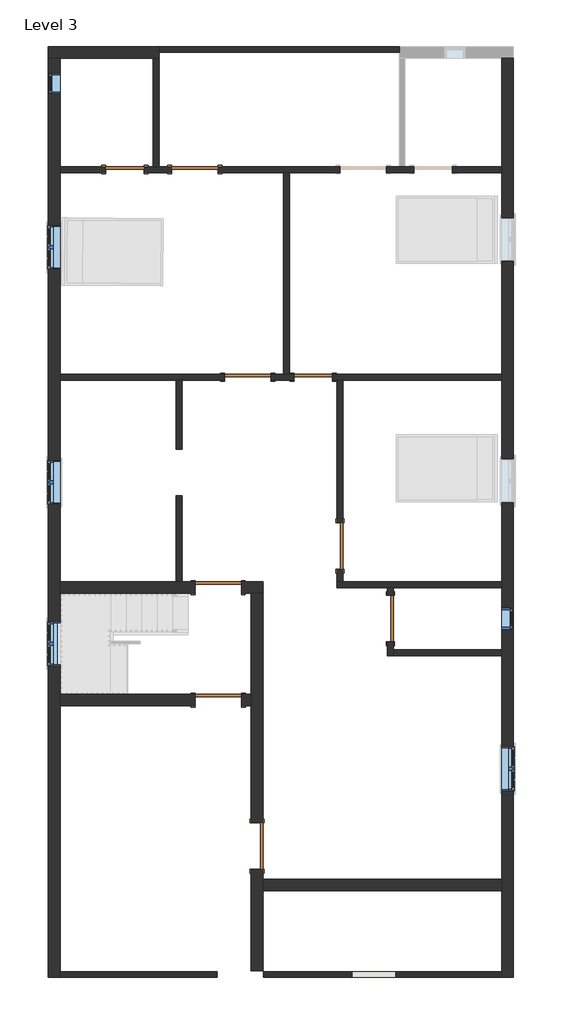
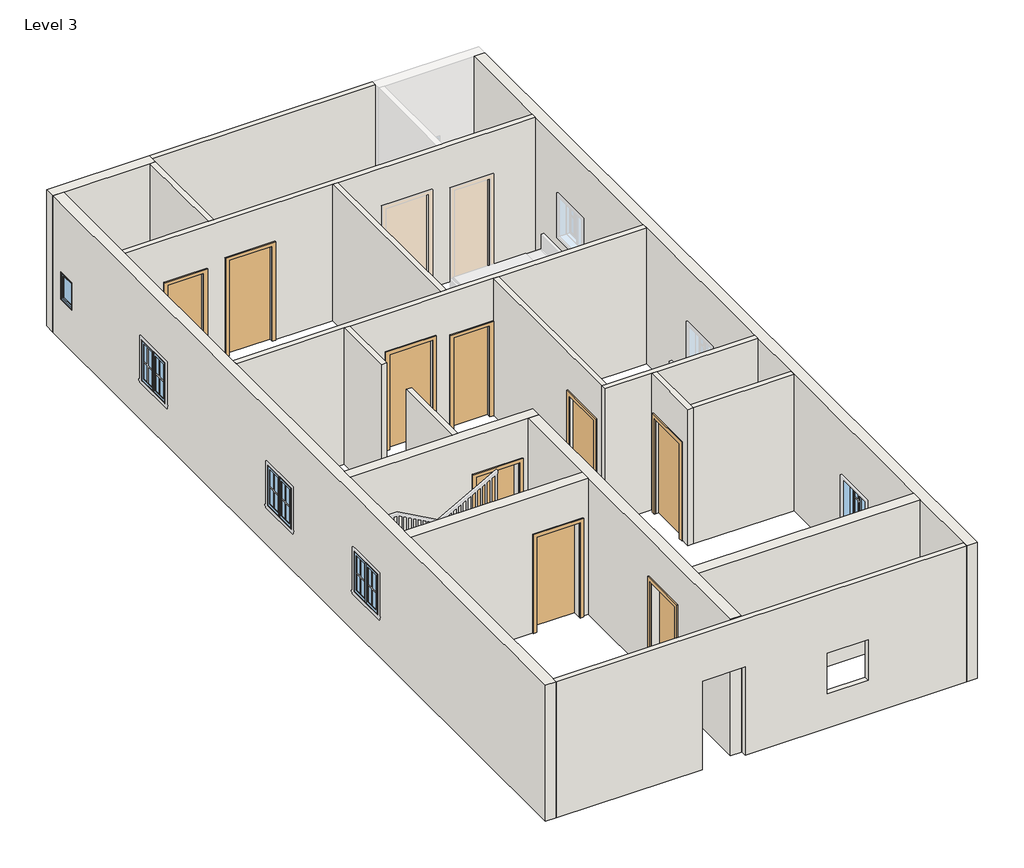
# One storey, part 1 of 3: 19 walls, 9 doors, 6 windows.
"""IFC4 building model written with IfcOpenShell, lengths in millimetres."""

from ifc_helpers import new_model, si_unit, frame, origin, place, context, project, spatial, polyline, outline, extrude, faceted_brep, transform, mapped, element, save
from components import door_d8f5dbb5, door_f2b275c1, door_e5f9f3c4, door_0ca8825f, door_305aa2a5, window_aa618e30, window_339605e1

model = new_model("IFC4")

# Units and contexts
model_context = context("Model", 3, world=origin())
ifc_project = project(units=[si_unit("LENGTHUNIT", "METRE", prefix="MILLI")], contexts=[model_context])

# Site, building, storey
site = spatial("IfcSite", under=ifc_project)
building = spatial("IfcBuilding", under=site)
storey = spatial("IfcBuildingStorey", under=building, Name="Level 3", Elevation=3200.4)

# Doors
placement = place(None, origin())
door_shape = door_d8f5dbb5(model_context)
element("IfcDoor", 1, ObjectType="Single-Flush : 30\" x 80\"", at=placement, inside=storey, context=model_context, shape_type="MappedRepresentation", body=[
    mapped(door_shape, transform((-4322.2915084, 8007.7072267, 3200.4), x_axis=(1.0, 0.0, 0.0), y_axis=(0.0, 1.0, 0.0), z_axis=(0.0, 0.0, 1.0))),
])
door_2_shape = door_f2b275c1(model_context)
element("IfcDoor", 2, ObjectType="Single-Flush : 30\" x 80\"", at=placement, inside=storey, context=model_context, shape_type="MappedRepresentation", body=[
    mapped(door_2_shape, transform((-621.124692, 3931.0072267, 3200.4), x_axis=(-1.0, 0.0, 0.0), y_axis=(0.0, -1.0, 0.0), z_axis=(0.0, 0.0, 1.0))),
])
door_3_shape = door_e5f9f3c4(model_context)
element("IfcDoor", 3, ObjectType="Single-Flush : 36\" x 84\"", at=placement, inside=storey, context=model_context, shape_type="MappedRepresentation", body=[
    mapped(door_3_shape, transform((-1909.2915084, 3931.0072267, 3200.4), x_axis=(1.0, 0.0, 0.0), y_axis=(0.0, 1.0, 0.0), z_axis=(0.0, 0.0, 1.0))),
])
element("IfcDoor", 4, ObjectType="Single-Flush : 36\" x 84\"", at=placement, inside=storey, context=model_context, shape_type="MappedRepresentation", body=[
    mapped(door_3_shape, transform((-94.9578757, 616.3072267, 3200.4), x_axis=(0.0, -1.0, 0.0), y_axis=(1.0, 0.0, 0.0), z_axis=(0.0, 0.0, 1.0))),
])
door_4_shape = door_0ca8825f(model_context)
element("IfcDoor", 5, ObjectType="Single-Flush : 36\" x 84\"", at=placement, inside=storey, context=model_context, shape_type="MappedRepresentation", body=[
    mapped(door_4_shape, transform((-2490.3165084, -202.8427733, 3200.4), x_axis=(1.0, 0.0, 0.0), y_axis=(0.0, 1.0, 0.0), z_axis=(0.0, 0.0, 1.0))),
])
element("IfcDoor", 6, ObjectType="Single-Flush : 36\" x 84\"", at=placement, inside=storey, context=model_context, shape_type="MappedRepresentation", body=[
    mapped(door_4_shape, transform((-2487.1415084, -2412.6427733, 3200.4), x_axis=(1.0, 0.0, 0.0), y_axis=(0.0, 1.0, 0.0), z_axis=(0.0, 0.0, 1.0))),
])
element("IfcDoor", 7, ObjectType="Single-Flush : 36\" x 84\"", at=placement, inside=storey, context=model_context, shape_type="MappedRepresentation", body=[
    mapped(door_4_shape, transform((-1725.1415084, -5282.8427733, 3200.4), x_axis=(0.0, -1.0, 0.0), y_axis=(1.0, 0.0, 0.0), z_axis=(0.0, 0.0, 1.0))),
])
door_5_shape = door_305aa2a5(model_context)
element("IfcDoor", 8, ObjectType="Single-Flush : 36\" x 84\"", at=placement, inside=storey, context=model_context, shape_type="MappedRepresentation", body=[
    mapped(door_5_shape, transform((897.4084916, -812.4427733, 3200.4), x_axis=(0.0, 1.0, 0.0), y_axis=(-1.0, 0.0, 0.0), z_axis=(0.0, 0.0, 1.0))),
])
element("IfcDoor", 9, ObjectType="Single-Flush : 36\" x 84\"", at=placement, inside=storey, context=model_context, shape_type="MappedRepresentation", body=[
    mapped(door_5_shape, transform((-2950.6915084, 8007.7072267, 3200.4), x_axis=(-1.0, 0.0, 0.0), y_axis=(0.0, -1.0, 0.0), z_axis=(0.0, 0.0, 1.0))),
])

# Walls
element("IfcWall", 10, ObjectType="WALL4.5\"", at=placement, inside=storey, context=model_context, shape_type="Brep", body=[
    faceted_brep([(821.2084916, 7950.5572267, 5334.0), (821.2084916, 7950.5572267, 3200.4), (1354.6084916, 7950.5572267, 3200.4), (1354.6084916, 7950.5572267, 5232.4), (2116.6084916, 7950.5572267, 5232.4), (2116.6084916, 7950.5572267, 3200.4), (3088.1584916, 7950.5572267, 3200.4), (3088.1584916, 7950.5572267, 6248.4), (-1090.1415084, 7950.5572267, 6248.4), (-1204.4415084, 7950.5572267, 6248.4), (-5598.6415084, 7950.5572267, 6248.4), (-5598.6415084, 7950.5572267, 3200.4), (-4703.2915084, 7950.5572267, 3200.4), (-4703.2915084, 7950.5572267, 5232.4), (-3941.2915084, 7950.5572267, 5232.4), (-3941.2915084, 7950.5572267, 3200.4), (-3407.8915084, 7950.5572267, 3200.4), (-3407.8915084, 7950.5572267, 5334.0), (-2493.4915084, 7950.5572267, 5334.0), (-2493.4915084, 7950.5572267, 3200.4), (-1204.4415084, 7950.5572267, 3200.4), (-1090.1415084, 7950.5572267, 3200.4), (-93.1915084, 7950.5572267, 3200.4), (-93.1915084, 7950.5572267, 5334.0), (1354.6084916, 8064.8572267, 3200.4), (1183.1584916, 8064.8572267, 3200.4), (1068.8584916, 8064.8572267, 3200.4), (821.2084916, 8064.8572267, 3200.4), (821.2084916, 8064.8572267, 5334.0), (-93.1915084, 8064.8572267, 5334.0), (-93.1915084, 8064.8572267, 3200.4), (-2493.4915084, 8064.8572267, 3200.4), (-2493.4915084, 8064.8572267, 5334.0), (-3407.8915084, 8064.8572267, 5334.0), (-3407.8915084, 8064.8572267, 3200.4), (-3655.5415084, 8064.8572267, 3200.4), (-3769.8415084, 8064.8572267, 3200.4), (-3941.2915084, 8064.8572267, 3200.4), (-3941.2915084, 8064.8572267, 5232.4), (-4703.2915084, 8064.8572267, 5232.4), (-4703.2915084, 8064.8572267, 3200.4), (-5598.6415084, 8064.8572267, 3200.4), (-5598.6415084, 8064.8572267, 6248.4), (-3769.8415084, 8064.8572267, 6248.4), (-3655.5415084, 8064.8572267, 6248.4), (1068.8584916, 8064.8572267, 6248.4), (1183.1584916, 8064.8572267, 6248.4), (3088.1584916, 8064.8572267, 6248.4), (3088.1584916, 8064.8572267, 3200.4), (2116.6084916, 8064.8572267, 3200.4), (2116.6084916, 8064.8572267, 5232.4), (1354.6084916, 8064.8572267, 5232.4)], [[[0, 1, 2, 3, 4, 5, 6, 7, 8, 9, 10, 11, 12, 13, 14, 15, 16, 17, 18, 19, 20, 21, 22, 23]], [[24, 25, 26, 27, 28, 29, 30, 31, 32, 33, 34, 35, 36, 37, 38, 39, 40, 41, 42, 43, 44, 45, 46, 47, 48, 49, 50, 51]], [[12, 11, 41, 40]], [[49, 48, 6, 5]], [[37, 36, 35, 34, 16, 15]], [[2, 1, 27, 26, 25, 24]], [[22, 21, 20, 19, 31, 30]], [[11, 10, 42, 41]], [[7, 6, 48, 47]], [[38, 37, 15, 14]], [[39, 38, 14, 13]], [[40, 39, 13, 12]], [[3, 2, 24, 51]], [[4, 3, 51, 50]], [[5, 4, 50, 49]], [[17, 16, 34, 33]], [[18, 17, 33, 32]], [[19, 18, 32, 31]], [[28, 27, 1, 0]], [[29, 28, 0, 23]], [[30, 29, 23, 22]], [[10, 9, 8, 7, 47, 46, 45, 44, 43, 42]]]),
])
element("IfcWall", 11, ObjectType="WALL4.5\"", at=placement, inside=storey, context=model_context, shape_type="SweptSolid", body=[
    extrude(outline(polyline([(-3769.8415084, 8064.8572267), (-3769.8415084, 10198.4572267), (-3655.5415084, 10198.4572267), (-3655.5415084, 8064.8572267), (-3769.8415084, 8064.8572267)])), frame((0.0, 0.0, 3200.4), z_axis=(0.0, 0.0, 1.0), x_axis=(1.0, 0.0, 0.0)), (0.0, 0.0, 1.0), 3048.0),
])
element("IfcWall", 12, ObjectType="WALL4.5\"", at=placement, inside=storey, context=model_context, shape_type="SweptSolid", body=[
    extrude(outline(polyline([(-1204.4415084, 3988.1572267), (-1204.4415084, 7950.5572267), (-1090.1415084, 7950.5572267), (-1090.1415084, 3988.1572267), (-1204.4415084, 3988.1572267)])), frame((0.0, 0.0, 3200.4), z_axis=(0.0, 0.0, 1.0), x_axis=(1.0, 0.0, 0.0)), (0.0, 0.0, 1.0), 3048.0),
])
element("IfcWall", 13, ObjectType="WALL4.5\"", at=placement, inside=storey, context=model_context, shape_type="Brep", body=[
    faceted_brep([(-1452.0915084, 3873.8572267, 3200.4), (-1002.124692, 3873.8572267, 3200.4), (-1002.124692, 3873.8572267, 5232.4), (-240.124692, 3873.8572267, 5232.4), (-240.124692, 3873.8572267, 3200.4), (-152.1078757, 3873.8572267, 3200.4), (-37.8078757, 3873.8572267, 3200.4), (3088.1584916, 3873.8572267, 3200.4), (3088.1584916, 3873.8572267, 6248.4), (-37.8078757, 3873.8572267, 6248.4), (-152.1078757, 3873.8572267, 6248.4), (-3198.3415084, 3873.8572267, 6248.4), (-3312.6415084, 3873.8572267, 6248.4), (-5598.6415084, 3873.8572267, 6248.4), (-5598.6415084, 3873.8572267, 3200.4), (-3312.6415084, 3873.8572267, 3200.4), (-3198.3415084, 3873.8572267, 3200.4), (-2366.4915084, 3873.8572267, 3200.4), (-2366.4915084, 3873.8572267, 5334.0), (-1452.0915084, 3873.8572267, 5334.0), (-1002.124692, 3988.1572267, 5232.4), (-1002.124692, 3988.1572267, 3200.4), (-1090.1415084, 3988.1572267, 3200.4), (-1204.4415084, 3988.1572267, 3200.4), (-1452.0915084, 3988.1572267, 3200.4), (-1452.0915084, 3988.1572267, 5334.0), (-2366.4915084, 3988.1572267, 5334.0), (-2366.4915084, 3988.1572267, 3200.4), (-5598.6415084, 3988.1572267, 3200.4), (-5598.6415084, 3988.1572267, 6248.4), (-1204.4415084, 3988.1572267, 6248.4), (-1090.1415084, 3988.1572267, 6248.4), (3088.1584916, 3988.1572267, 6248.4), (3088.1584916, 3988.1572267, 3200.4), (-240.124692, 3988.1572267, 3200.4), (-240.124692, 3988.1572267, 5232.4)], [[[0, 1, 2, 3, 4, 5, 6, 7, 8, 9, 10, 11, 12, 13, 14, 15, 16, 17, 18, 19]], [[20, 21, 22, 23, 24, 25, 26, 27, 28, 29, 30, 31, 32, 33, 34, 35]], [[17, 16, 15, 14, 28, 27]], [[34, 33, 7, 6, 5, 4]], [[24, 23, 22, 21, 1, 0]], [[14, 13, 29, 28]], [[8, 7, 33, 32]], [[25, 24, 0, 19]], [[26, 25, 19, 18]], [[27, 26, 18, 17]], [[2, 1, 21, 20]], [[3, 2, 20, 35]], [[4, 3, 35, 34]], [[13, 12, 11, 10, 9, 8, 32, 31, 30, 29]]]),
])
element("IfcWall", 14, ObjectType="WALL4.5\"", at=placement, inside=storey, context=model_context, shape_type="SweptSolid", body=[
    extrude(outline(polyline([(-3312.6415084, 2514.5843832), (-3312.6415084, 3873.8572267), (-3198.3415084, 3873.8572267), (-3198.3415084, 2514.5843832), (-3312.6415084, 2514.5843832)])), frame((0.0, 0.0, 3200.4), z_axis=(0.0, 0.0, 1.0), x_axis=(1.0, 0.0, 0.0)), (0.0, 0.0, 1.0), 3048.0),
])
element("IfcWall", 15, ObjectType="WALL4.5\"", at=placement, inside=storey, context=model_context, shape_type="SweptSolid", body=[
    extrude(outline(polyline([(-3312.6415084, -88.5427733), (-3312.6415084, 1600.2092553), (-3198.3415084, 1600.2092553), (-3198.3415084, -88.5427733), (-3312.6415084, -88.5427733)])), frame((0.0, 0.0, 3200.4), z_axis=(0.0, 0.0, 1.0), x_axis=(1.0, 0.0, 0.0)), (0.0, 0.0, 1.0), 3048.0),
])
element("IfcWall", 16, ObjectType="WALL4.5\"", at=placement, inside=storey, context=model_context, shape_type="SweptSolid", body=[
    extrude(outline(polyline([(159.1072267, 5334.0), (159.1072267, 3200.4), (-88.5427733, 3200.4), (-88.5427733, 6248.4), (3873.8572267, 6248.4), (3873.8572267, 3200.4), (1073.5072267, 3200.4), (1073.5072267, 5334.0), (159.1072267, 5334.0)])), frame((-152.1078757, 0.0, 0.0), z_axis=(1.0, 0.0, 0.0), x_axis=(0.0, 1.0, 0.0)), (0.0, 0.0, 1.0), 114.3),
])
element("IfcWall", 17, ObjectType="WALL4.5\"", at=placement, inside=storey, context=model_context, shape_type="Brep", body=[
    faceted_brep([(-152.1078757, -202.8427733, 3200.4), (840.2584916, -202.8427733, 3200.4), (954.5584916, -202.8427733, 3200.4), (3088.1584916, -202.8427733, 3200.4), (3088.1584916, -202.8427733, 6248.4), (954.5584916, -202.8427733, 6248.4), (840.2584916, -202.8427733, 6248.4), (-152.1078757, -202.8427733, 6248.4), (-152.1078757, -88.5427733, 3200.4), (-152.1078757, -88.5427733, 6248.4), (-37.8078757, -88.5427733, 6248.4), (3088.1584916, -88.5427733, 6248.4), (3088.1584916, -88.5427733, 3200.4), (-37.8078757, -88.5427733, 3200.4)], [[[0, 1, 2, 3, 4, 5, 6, 7]], [[8, 9, 10, 11, 12, 13]], [[3, 2, 1, 0, 8, 13, 12]], [[4, 3, 12, 11]], [[0, 7, 9, 8]], [[7, 6, 5, 4, 11, 10, 9]]]),
])
element("IfcWall", 18, ObjectType="WALL4.5\"", at=placement, inside=storey, context=model_context, shape_type="Brep", body=[
    faceted_brep([(840.2584916, -202.8427733, 3200.4), (840.2584916, -355.2427733, 3200.4), (840.2584916, -355.2427733, 5334.0), (840.2584916, -1269.6427733, 5334.0), (840.2584916, -1269.6427733, 3200.4), (840.2584916, -1536.3427733, 3200.4), (840.2584916, -1536.3427733, 6248.4), (840.2584916, -202.8427733, 6248.4), (954.5584916, -355.2427733, 5334.0), (954.5584916, -355.2427733, 3200.4), (954.5584916, -202.8427733, 3200.4), (954.5584916, -202.8427733, 6248.4), (954.5584916, -1422.0427733, 6248.4), (954.5584916, -1536.3427733, 6248.4), (954.5584916, -1536.3427733, 3200.4), (954.5584916, -1422.0427733, 3200.4), (954.5584916, -1269.6427733, 3200.4), (954.5584916, -1269.6427733, 5334.0)], [[[0, 1, 2, 3, 4, 5, 6, 7]], [[8, 9, 10, 11, 12, 13, 14, 15, 16, 17]], [[10, 9, 1, 0]], [[16, 15, 14, 5, 4]], [[0, 7, 11, 10]], [[6, 5, 14, 13]], [[2, 1, 9, 8]], [[3, 2, 8, 17]], [[4, 3, 17, 16]], [[7, 6, 13, 12, 11]]]),
])
element("IfcWall", 19, ObjectType="WALL4.5\"", at=placement, inside=storey, context=model_context, shape_type="SweptSolid", body=[
    extrude(outline(polyline([(3088.1584916, -1536.3427733), (954.5584916, -1536.3427733), (954.5584916, -1422.0427733), (3088.1584916, -1422.0427733), (3088.1584916, -1536.3427733)])), frame((0.0, 0.0, 3200.4), z_axis=(0.0, 0.0, 1.0), x_axis=(1.0, 0.0, 0.0)), (0.0, 0.0, 1.0), 3048.0),
])
element("IfcWall", 20, ObjectType="WALL4.5\"", at=placement, inside=storey, context=model_context, shape_type="SweptSolid", body=[
    extrude(outline(polyline([(6248.4, -5598.6415084), (3200.4, -5598.6415084), (3200.4, -2512.5415084), (5181.6, -2512.5415084), (5181.6, -1598.1415084), (3200.4, -1598.1415084), (3200.4, 3088.1584916), (6248.4, 3088.1584916), (6248.4, -5598.6415084)]), holes=[polyline([(4876.8, 141.7584916), (4876.8, 1005.3584916), (3962.4, 1005.3584916), (3962.4, 141.7584916), (4876.8, 141.7584916)])]), frame((0.0, -7860.9427733, 0.0), z_axis=(0.0, 1.0, 0.0), x_axis=(0.0, 0.0, 1.0)), (0.0, 0.0, 1.0), 114.3),
])
element("IfcWall", 21, ObjectType="WALL4.5\"", at=placement, inside=storey, context=model_context, shape_type="SweptSolid", body=[
    extrude(outline(polyline([(1068.8584916, 10312.7572267), (-3655.5415084, 10312.7572267), (-3655.5415084, 10427.0572267), (1068.8584916, 10427.0572267), (1068.8584916, 10312.7572267)])), frame((0.0, 0.0, 3200.4), z_axis=(0.0, 0.0, 1.0), x_axis=(1.0, 0.0, 0.0)), (0.0, 0.0, 1.0), 3048.0),
])
element("IfcWall", 22, ObjectType="WALL9\"", at=placement, inside=storey, context=model_context, shape_type="Brep", body=[
    faceted_brep([(-3655.5415084, 10427.0572267, 3200.4), (-5827.2415084, 10427.0572267, 3200.4), (-5827.2415084, 10427.0572267, 6248.4), (-3655.5415084, 10427.0572267, 6248.4), (-3655.5415084, 10198.4572267, 3200.4), (-3655.5415084, 10198.4572267, 6248.4), (-3769.8415084, 10198.4572267, 6248.4), (-5598.6415084, 10198.4572267, 6248.4), (-5827.2415084, 10198.4572267, 6248.4), (-5827.2415084, 10198.4572267, 3200.4), (-5598.6415084, 10198.4572267, 3200.4), (-3769.8415084, 10198.4572267, 3200.4), (-3655.5415084, 10312.7572267, 3200.4), (-3655.5415084, 10312.7572267, 6248.4)], [[[0, 1, 2, 3]], [[4, 5, 6, 7, 8, 9, 10, 11]], [[1, 0, 12, 4, 11, 10, 9]], [[2, 1, 9, 8]], [[0, 3, 13, 5, 4, 12]], [[3, 2, 8, 7, 6, 5, 13]]]),
])
element("IfcWall", 23, ObjectType="WALL9\"", at=placement, inside=storey, context=model_context, shape_type="Brep", body=[
    faceted_brep([(-5827.2415084, 10198.4572267, 3200.4), (-5827.2415084, -7860.9427733, 3200.4), (-5827.2415084, -7860.9427733, 6248.4), (-5827.2415084, 10198.4572267, 6248.4), (-5827.2415084, 9906.3572267, 4724.4), (-5827.2415084, 9499.9572267, 4724.4), (-5827.2415084, 9499.9572267, 4114.8), (-5827.2415084, 9906.3572267, 4114.8), (-5827.2415084, 6915.5072267, 5029.2), (-5827.2415084, 6051.9072267, 5029.2), (-5827.2415084, 6051.9072267, 4114.8), (-5827.2415084, 6915.5072267, 4114.8), (-5827.2415084, 2295.8822267, 5029.2), (-5827.2415084, 1432.2822267, 5029.2), (-5827.2415084, 1432.2822267, 4114.8), (-5827.2415084, 2295.8822267, 4114.8), (-5827.2415084, -875.9427733, 5029.2), (-5827.2415084, -1739.5427733, 5029.2), (-5827.2415084, -1739.5427733, 4114.8), (-5827.2415084, -875.9427733, 4114.8), (-5598.6415084, 10198.4572267, 3200.4), (-5598.6415084, 10198.4572267, 6248.4), (-5598.6415084, 8064.8572267, 6248.4), (-5598.6415084, 7950.5572267, 6248.4), (-5598.6415084, 3988.1572267, 6248.4), (-5598.6415084, 3873.8572267, 6248.4), (-5598.6415084, -88.5427733, 6248.4), (-5598.6415084, -317.1427733, 6248.4), (-5598.6415084, -2298.3427733, 6248.4), (-5598.6415084, -2526.9427733, 6248.4), (-5598.6415084, -7746.6427733, 6248.4), (-5598.6415084, -7860.9427733, 6248.4), (-5598.6415084, -7860.9427733, 3200.4), (-5598.6415084, -7746.6427733, 3200.4), (-5598.6415084, -2526.9427733, 3200.4), (-5598.6415084, -2298.3427733, 3200.4), (-5598.6415084, -317.1427733, 3200.4), (-5598.6415084, -88.5427733, 3200.4), (-5598.6415084, 3873.8572267, 3200.4), (-5598.6415084, 3988.1572267, 3200.4), (-5598.6415084, 7950.5572267, 3200.4), (-5598.6415084, 8064.8572267, 3200.4), (-5598.6415084, 9906.3572267, 4724.4), (-5598.6415084, 9906.3572267, 4114.8), (-5598.6415084, 9499.9572267, 4114.8), (-5598.6415084, 9499.9572267, 4724.4), (-5598.6415084, 6915.5072267, 5029.2), (-5598.6415084, 6915.5072267, 4114.8), (-5598.6415084, 6051.9072267, 4114.8), (-5598.6415084, 6051.9072267, 5029.2), (-5598.6415084, 2295.8822267, 5029.2), (-5598.6415084, 2295.8822267, 4114.8), (-5598.6415084, 1432.2822267, 4114.8), (-5598.6415084, 1432.2822267, 5029.2), (-5598.6415084, -875.9427733, 5029.2), (-5598.6415084, -875.9427733, 4114.8), (-5598.6415084, -1739.5427733, 4114.8), (-5598.6415084, -1739.5427733, 5029.2)], [[[0, 1, 2, 3], [4, 5, 6, 7], [8, 9, 10, 11], [12, 13, 14, 15], [16, 17, 18, 19]], [[20, 21, 22, 23, 24, 25, 26, 27, 28, 29, 30, 31, 32, 33, 34, 35, 36, 37, 38, 39, 40, 41], [42, 43, 44, 45], [46, 47, 48, 49], [50, 51, 52, 53], [54, 55, 56, 57]], [[1, 0, 20, 41, 40, 39, 38, 37, 36, 35, 34, 33, 32]], [[0, 3, 21, 20]], [[2, 1, 32, 31]], [[43, 42, 4, 7]], [[44, 43, 7, 6]], [[45, 44, 6, 5]], [[42, 45, 5, 4]], [[47, 46, 8, 11]], [[48, 47, 11, 10]], [[49, 48, 10, 9]], [[46, 49, 9, 8]], [[51, 50, 12, 15]], [[52, 51, 15, 14]], [[53, 52, 14, 13]], [[50, 53, 13, 12]], [[55, 54, 16, 19]], [[56, 55, 19, 18]], [[57, 56, 18, 17]], [[54, 57, 17, 16]], [[3, 2, 31, 30, 29, 28, 27, 26, 25, 24, 23, 22, 21]]]),
])
element("IfcWall", 24, ObjectType="WALL9\"", at=placement, inside=storey, context=model_context, shape_type="Brep", body=[
    faceted_brep([(3088.1584916, 10198.4572267, 3200.4), (3088.1584916, 8064.8572267, 3200.4), (3088.1584916, 7950.5572267, 3200.4), (3088.1584916, 3988.1572267, 3200.4), (3088.1584916, 3873.8572267, 3200.4), (3088.1584916, -88.5427733, 3200.4), (3088.1584916, -202.8427733, 3200.4), (3088.1584916, -1422.0427733, 3200.4), (3088.1584916, -1536.3427733, 3200.4), (3088.1584916, -5930.5427733, 3200.4), (3088.1584916, -6159.1427733, 3200.4), (3088.1584916, -7746.6427733, 3200.4), (3088.1584916, -7860.9427733, 3200.4), (3088.1584916, -7860.9427733, 6248.4), (3088.1584916, -7746.6427733, 6248.4), (3088.1584916, -6159.1427733, 6248.4), (3088.1584916, -5930.5427733, 6248.4), (3088.1584916, -1536.3427733, 6248.4), (3088.1584916, -1422.0427733, 6248.4), (3088.1584916, -202.8427733, 6248.4), (3088.1584916, -88.5427733, 6248.4), (3088.1584916, 3873.8572267, 6248.4), (3088.1584916, 3988.1572267, 6248.4), (3088.1584916, 7950.5572267, 6248.4), (3088.1584916, 8064.8572267, 6248.4), (3088.1584916, 10198.4572267, 6248.4), (3088.1584916, -1015.6427733, 4724.4), (3088.1584916, -1015.6427733, 4114.8), (3088.1584916, -609.2427733, 4114.8), (3088.1584916, -609.2427733, 4724.4), (3088.1584916, 6204.3072267, 5029.2), (3088.1584916, 6204.3072267, 4114.8), (3088.1584916, 7067.9072267, 4114.8), (3088.1584916, 7067.9072267, 5029.2), (3088.1584916, 1460.8572267, 5029.2), (3088.1584916, 1460.8572267, 4114.8), (3088.1584916, 2324.4572267, 4114.8), (3088.1584916, 2324.4572267, 5029.2), (3088.1584916, -4193.8177733, 5029.2), (3088.1584916, -4193.8177733, 4114.8), (3088.1584916, -3330.2177733, 4114.8), (3088.1584916, -3330.2177733, 5029.2), (3316.7584916, 10198.4572267, 3200.4), (3316.7584916, 10198.4572267, 6248.4), (3316.7584916, -7860.9427733, 6248.4), (3316.7584916, -7860.9427733, 3200.4), (3316.7584916, -1015.6427733, 4724.4), (3316.7584916, -609.2427733, 4724.4), (3316.7584916, -609.2427733, 4114.8), (3316.7584916, -1015.6427733, 4114.8), (3316.7584916, 6204.3072267, 5029.2), (3316.7584916, 7067.9072267, 5029.2), (3316.7584916, 7067.9072267, 4114.8), (3316.7584916, 6204.3072267, 4114.8), (3316.7584916, 1460.8572267, 5029.2), (3316.7584916, 2324.4572267, 5029.2), (3316.7584916, 2324.4572267, 4114.8), (3316.7584916, 1460.8572267, 4114.8), (3316.7584916, -4193.8177733, 5029.2), (3316.7584916, -3330.2177733, 5029.2), (3316.7584916, -3330.2177733, 4114.8), (3316.7584916, -4193.8177733, 4114.8)], [[[0, 1, 2, 3, 4, 5, 6, 7, 8, 9, 10, 11, 12, 13, 14, 15, 16, 17, 18, 19, 20, 21, 22, 23, 24, 25], [26, 27, 28, 29], [30, 31, 32, 33], [34, 35, 36, 37], [38, 39, 40, 41]], [[42, 43, 44, 45], [46, 47, 48, 49], [50, 51, 52, 53], [54, 55, 56, 57], [58, 59, 60, 61]], [[12, 11, 10, 9, 8, 7, 6, 5, 4, 3, 2, 1, 0, 42, 45]], [[0, 25, 43, 42]], [[13, 12, 45, 44]], [[27, 26, 46, 49]], [[28, 27, 49, 48]], [[29, 28, 48, 47]], [[26, 29, 47, 46]], [[31, 30, 50, 53]], [[32, 31, 53, 52]], [[33, 32, 52, 51]], [[30, 33, 51, 50]], [[35, 34, 54, 57]], [[36, 35, 57, 56]], [[37, 36, 56, 55]], [[34, 37, 55, 54]], [[39, 38, 58, 61]], [[40, 39, 61, 60]], [[41, 40, 60, 59]], [[38, 41, 59, 58]], [[25, 24, 23, 22, 21, 20, 19, 18, 17, 16, 15, 14, 13, 44, 43]]]),
])
element("IfcWall", 25, ObjectType="WALL9\"", at=placement, inside=storey, context=model_context, shape_type="Brep", body=[
    faceted_brep([(-2033.1165084, -317.1427733, 5334.0), (-2033.1165084, -317.1427733, 3200.4), (-1839.4415084, -317.1427733, 3200.4), (-1610.8415084, -317.1427733, 3200.4), (-1610.8415084, -317.1427733, 6248.4), (-1839.4415084, -317.1427733, 6248.4), (-5598.6415084, -317.1427733, 6248.4), (-5598.6415084, -317.1427733, 3200.4), (-2947.5165084, -317.1427733, 3200.4), (-2947.5165084, -317.1427733, 5334.0), (-1610.8415084, -88.5427733, 3200.4), (-2033.1165084, -88.5427733, 3200.4), (-2033.1165084, -88.5427733, 5334.0), (-2947.5165084, -88.5427733, 5334.0), (-2947.5165084, -88.5427733, 3200.4), (-3198.3415084, -88.5427733, 3200.4), (-3312.6415084, -88.5427733, 3200.4), (-5598.6415084, -88.5427733, 3200.4), (-5598.6415084, -88.5427733, 6248.4), (-3312.6415084, -88.5427733, 6248.4), (-3198.3415084, -88.5427733, 6248.4), (-1610.8415084, -88.5427733, 6248.4)], [[[0, 1, 2, 3, 4, 5, 6, 7, 8, 9]], [[10, 11, 12, 13, 14, 15, 16, 17, 18, 19, 20, 21]], [[8, 7, 17, 16, 15, 14]], [[3, 2, 1, 11, 10]], [[7, 6, 18, 17]], [[4, 3, 10, 21]], [[12, 11, 1, 0]], [[13, 12, 0, 9]], [[14, 13, 9, 8]], [[6, 5, 4, 21, 20, 19, 18]]]),
])
element("IfcWall", 26, ObjectType="WALL9\"", at=placement, inside=storey, context=model_context, shape_type="Brep", body=[
    faceted_brep([(-1839.4415084, -5740.0427733, 5334.0), (-1839.4415084, -5740.0427733, 3200.4), (-1839.4415084, -7733.9427733, 3200.4), (-1839.4415084, -7733.9427733, 6248.4), (-1839.4415084, -2526.9427733, 6248.4), (-1839.4415084, -2298.3427733, 6248.4), (-1839.4415084, -317.1427733, 6248.4), (-1839.4415084, -317.1427733, 3200.4), (-1839.4415084, -2298.3427733, 3200.4), (-1839.4415084, -2526.9427733, 3200.4), (-1839.4415084, -4825.6427733, 3200.4), (-1839.4415084, -4825.6427733, 5334.0), (-1610.8415084, -7733.9427733, 3200.4), (-1610.8415084, -6159.1427733, 3200.4), (-1610.8415084, -5930.5427733, 3200.4), (-1610.8415084, -5740.0427733, 3200.4), (-1610.8415084, -5740.0427733, 5334.0), (-1610.8415084, -4825.6427733, 5334.0), (-1610.8415084, -4825.6427733, 3200.4), (-1610.8415084, -317.1427733, 3200.4), (-1610.8415084, -317.1427733, 6248.4), (-1610.8415084, -5930.5427733, 6248.4), (-1610.8415084, -6159.1427733, 6248.4), (-1610.8415084, -7733.9427733, 6248.4)], [[[0, 1, 2, 3, 4, 5, 6, 7, 8, 9, 10, 11]], [[12, 13, 14, 15, 16, 17, 18, 19, 20, 21, 22, 23]], [[2, 1, 15, 14, 13, 12]], [[10, 9, 8, 7, 19, 18]], [[3, 2, 12, 23]], [[7, 6, 20, 19]], [[16, 15, 1, 0]], [[17, 16, 0, 11]], [[18, 17, 11, 10]], [[6, 5, 4, 3, 23, 22, 21, 20]]]),
])
element("IfcWall", 27, ObjectType="WALL9\"", at=placement, inside=storey, context=model_context, shape_type="SweptSolid", body=[
    extrude(outline(polyline([(3088.1584916, -6159.1427733), (-1610.8415084, -6159.1427733), (-1610.8415084, -5930.5427733), (3088.1584916, -5930.5427733), (3088.1584916, -6159.1427733)])), frame((0.0, 0.0, 3200.4), z_axis=(0.0, 0.0, 1.0), x_axis=(1.0, 0.0, 0.0)), (0.0, 0.0, 1.0), 3048.0),
])
element("IfcWall", 28, ObjectType="WALL9\"", at=placement, inside=storey, context=model_context, shape_type="SweptSolid", body=[
    extrude(outline(polyline([(5334.0, -2029.9415084), (3200.4, -2029.9415084), (3200.4, -1839.4415084), (6248.4, -1839.4415084), (6248.4, -5598.6415084), (3200.4, -5598.6415084), (3200.4, -2944.3415084), (5334.0, -2944.3415084), (5334.0, -2029.9415084)])), frame((0.0, -2526.9427733, 0.0), z_axis=(0.0, 1.0, 0.0), x_axis=(0.0, 0.0, 1.0)), (0.0, 0.0, 1.0), 228.6),
])

# Windows
window_shape = window_aa618e30(model_context)
element("IfcWindow", 29, ObjectType="Fixed : 16\" x 24\"", at=placement, inside=storey, context=model_context, shape_type="MappedRepresentation", body=[
    mapped(window_shape, transform((-5712.9415084, 9741.2572267, 3200.4), x_axis=(0.0, 1.0, 0.0), y_axis=(-1.0, 0.0, 0.0), z_axis=(0.0, 0.0, 1.0))),
])
element("IfcWindow", 30, ObjectType="Fixed : 16\" x 24\"", at=placement, inside=storey, context=model_context, shape_type="MappedRepresentation", body=[
    mapped(window_shape, transform((3202.4584916, -850.5427733, 3200.4), x_axis=(0.0, -1.0, 0.0), y_axis=(1.0, 0.0, 0.0), z_axis=(0.0, 0.0, 1.0))),
])
window_2_shape = window_339605e1(model_context)
element("IfcWindow", 31, ObjectType="Window-Casement-Double : 34\" x 36\"", at=placement, inside=storey, context=model_context, shape_type="MappedRepresentation", body=[
    mapped(window_2_shape, transform((-5712.9415084, 6483.7072267, 3200.4), x_axis=(0.0, 1.0, 0.0), y_axis=(-1.0, 0.0, 0.0), z_axis=(0.0, 0.0, 1.0))),
])
element("IfcWindow", 32, ObjectType="Window-Casement-Double : 34\" x 36\"", at=placement, inside=storey, context=model_context, shape_type="MappedRepresentation", body=[
    mapped(window_2_shape, transform((-5712.9415084, 1864.0822267, 3200.4), x_axis=(0.0, 1.0, 0.0), y_axis=(-1.0, 0.0, 0.0), z_axis=(0.0, 0.0, 1.0))),
])
element("IfcWindow", 33, ObjectType="Window-Casement-Double : 34\" x 36\"", at=placement, inside=storey, context=model_context, shape_type="MappedRepresentation", body=[
    mapped(window_2_shape, transform((3202.4584916, -3762.0177733, 3200.4), x_axis=(0.0, -1.0, 0.0), y_axis=(1.0, 0.0, 0.0), z_axis=(0.0, 0.0, 1.0))),
])
element("IfcWindow", 34, ObjectType="Window-Casement-Double : 34\" x 36\"", at=placement, inside=storey, context=model_context, shape_type="MappedRepresentation", body=[
    mapped(window_2_shape, transform((-5712.9415084, -1307.7427733, 3200.4), x_axis=(0.0, 1.0, 0.0), y_axis=(-1.0, 0.0, 0.0), z_axis=(0.0, 0.0, 1.0))),
])

save(model, "model.ifc")

# Revit data of these elements
# Type "Single-Flush : 30\" x 80\""
#   Type Mark = "5"
#   Construction Type Id = "MDOOR"
#   Assembly Code = "C1020"
#   Analytic Construction = "Metal"
#   Thickness = 0' - 2"
#   Heat Transfer Coefficient (U) = 0.651978 BTU/(h·ft²·°F)
#   Height = 6' - 8"
#   Trim Projection Ext = 0' - 1"
#   Trim Projection Int = 0' - 1"
#   Trim Width = 0' - 3"
#   Width = 2' - 6"
#   Define Thermal Properties by = 1
#   Define Thermal Properties by = 1
#   Door Material = Door - Panel
#   Frame Material = Door - Frame
#   Visual Light Transmittance = 0
#   Solar Heat Gain Coefficient = 0
#   Function = (empty or 0)
#   Wall Closure = (empty or 0)
# Type "Single-Flush : 36\" x 84\""
#   Type Mark = "1"
#   Construction Type Id = "MDOOR"
#   Assembly Code = "C1020"
#   Analytic Construction = "Metal"
#   Thickness = 0' - 2"
#   Heat Transfer Coefficient (U) = 0.651978 BTU/(h·ft²·°F)
#   Height = 7' - 0"
#   Trim Projection Ext = 0' - 1"
#   Trim Projection Int = 0' - 1"
#   Trim Width = 0' - 3"
#   Width = 3' - 0"
#   Define Thermal Properties by = 1
#   Define Thermal Properties by = 1
#   Door Material = Door - Panel
#   Frame Material = Door - Frame
#   Visual Light Transmittance = 0
#   Solar Heat Gain Coefficient = 0
#   Function = (empty or 0)
#   Wall Closure = (empty or 0)
# Type "WALL4.5\""
#   Assembly Code = "B2010"
#   Layers, outside or top first: 0' - 4 1/2" no material (function 1)
# Type "WALL9\""
#   Assembly Code = "B2010"
#   Layers, outside or top first: 0' - 9" no material (function 1)
# Type "Fixed : 16\" x 24\""
#   Type Mark = "4"
#   Construction Type Id = "GSP4R"
#   Assembly Code = "B2020100"
#   Analytic Construction = "1/8 in Pilkington single glazing"
#   Visual Light Transmittance = 0.9
#   Solar Heat Gain Coefficient = 0.78
#   Heat Transfer Coefficient (U) = 0.6496 BTU/(h·ft²·°F)
#   Height = 2' - 0"
#   Default Sill Height = 3' - 0"
#   Width = 1' - 4"
#   Window Inset = 0' - 0 3/4"
#   Define Thermal Properties by = 1
#   Define Thermal Properties by = 1
#   Glass Pane Material = Glass
#   Sash Material = Sash
#   Wall Closure = (empty or 0)
# Type "Window-Casement-Double : 34\" x 36\""
#   Type Mark = "14"
#   Fire Rating = "0.5h"
#   Assembly Code = "B2020100"
#   Analytic Construction = "Double glazing - domestic"
#   Frame Extension [instance default] = 0' - 0 1/4"
#   Window Inset [instance default] = 0' - 0"
#   Wall Thickness [instance default] = 0' - 6"
#   Interior Wall Closure [instance default] = 0' - 2 1/4"
#   Half Width = 1' - 5"
#   Visual Light Transmittance = 0.81
#   Thermal Resistance (R) = 1.8146 (h·ft²·°F)/BTU
#   Solar Heat Gain Coefficient = 0.76
#   Rough Width = 2' - 10 1/2"
#   Rough Height = 3' - 0 1/2"
#   Height = 3' - 0"
#   Heat Transfer Coefficient (U) = 0.5511 BTU/(h·ft²·°F)
#   Exterior Wall Closure [instance default] = 0' - 1 1/4"
#   Extension Jamb [instance default] = 0' - 2 1/4"
#   Default Sill Height = 3' - 0"
#   Width = 2' - 10"
#   Define Thermal Properties by = 0
#   Muntin Visibility = yes
#   Interior Trim Visibility [instance default] = yes
#   Exterior Trim Visibility [instance default] = yes
#   Extension Jamb Visibility [instance default] = yes
#   Interior Trim Material = Wood - Stained
#   Muntin Pattern = Muntin Pattern_2x2 : Muntin Pattern_2x2
#   Interior Trim = Trim-Window-Interior-Flat : Picture Frame
#   Interior Frame Material = Wood - Stained
#   Glass Panel Material = Glass
#   Exterior Trim Material = Clad - White
#   Exterior Trim = Trim-Window-Exterior-Flat : with Sill
#   Exterior Frame Material = Clad - White
#   Wall Closure = (empty or 0)
# Elements 1, 2 (IfcDoor, "Single-Flush : 30\" x 80\"")
#   Phase Created = New Construction
#   Materials on its faces: "Door - Frame", "Door - Panel"
# Elements 3, 4, 5, 6, 7, 8, 9 (IfcDoor, "Single-Flush : 36\" x 84\"")
#   Phase Created = New Construction
#   Materials on its faces: "Door - Frame", "Door - Panel"
# Elements 10, 20, 21 (IfcWall, "WALL4.5\"")
#   Top Offset = 0' - 0"
#   Base Offset = 0' - 0"
#   Unconnected Height = 10' - 0"
#   wall height = 10' - 0"
#   Phase Created = New Construction
#   Base Constraint = Level 3
#   Materials on its faces: "Default Wall", "Wood Planks"
# Elements 11, 12, 13, 14, 15, 16, 17, 18, 19 (IfcWall, "WALL4.5\"")
#   Top Offset = 0' - 0"
#   Base Offset = 0' - 0"
#   Unconnected Height = 10' - 0"
#   wall height = 10' - 0"
#   Phase Created = New Construction
#   Base Constraint = Level 3
#   Materials on its faces: "Default Wall"
# Element 22 (IfcWall, "WALL9\"")
#   Top Offset = 0' - 0"
#   Base Offset = 0' - 0"
#   Unconnected Height = 10' - 0"
#   wall height = 10' - 0"
#   Phase Created = New Construction
#   Base Constraint = Level 3
#   Materials on its faces: "Wood Planks", "Default Wall"
# Elements 23, 24 (IfcWall, "WALL9\"")
#   Top Offset = 0' - 0"
#   Base Offset = 0' - 0"
#   Unconnected Height = 10' - 0"
#   wall height = 10' - 0"
#   Phase Created = New Construction
#   Base Constraint = Level 3
#   Materials on its faces: "Default Wall", "Wood Planks"
# Elements 25, 26, 27, 28 (IfcWall, "WALL9\"")
#   Top Offset = 0' - 0"
#   Base Offset = 0' - 0"
#   Unconnected Height = 10' - 0"
#   wall height = 10' - 0"
#   Phase Created = New Construction
#   Base Constraint = Level 3
#   Materials on its faces: "Default Wall"
# Element 29 (IfcWindow, "Fixed : 16\" x 24\"")
#   Mark = "10"
#   Phase Created = New Construction
#   Materials on its faces: "Sash", "Glass"
# Element 30 (IfcWindow, "Fixed : 16\" x 24\"")
#   Mark = "12"
#   Phase Created = New Construction
#   Materials on its faces: "Sash", "Glass"
# Element 31 (IfcWindow, "Window-Casement-Double : 34\" x 36\"")
#   Mark = "15"
#   Window Inset = 0' - 0"
#   Interior Wall Closure = 0' - 2 1/4"
#   Frame Extension = 0' - 0 1/4"
#   Exterior Wall Closure = 0' - 1 1/4"
#   Interior Trim Visibility = yes
#   Exterior Trim Visibility = yes
#   Phase Created = New Construction
#   Materials on its faces: "Wood - Stained", "Glass", "Clad - White"
# Element 32 (IfcWindow, "Window-Casement-Double : 34\" x 36\"")
#   Mark = "16"
#   Window Inset = 0' - 0"
#   Interior Wall Closure = 0' - 2 1/4"
#   Frame Extension = 0' - 0 1/4"
#   Exterior Wall Closure = 0' - 1 1/4"
#   Interior Trim Visibility = yes
#   Exterior Trim Visibility = yes
#   Phase Created = New Construction
#   Materials on its faces: "Wood - Stained", "Glass", "Clad - White"
# Element 33 (IfcWindow, "Window-Casement-Double : 34\" x 36\"")
#   Mark = "17"
#   Window Inset = 0' - 0"
#   Interior Wall Closure = 0' - 2 1/4"
#   Frame Extension = 0' - 0 1/4"
#   Exterior Wall Closure = 0' - 1 1/4"
#   Interior Trim Visibility = yes
#   Exterior Trim Visibility = yes
#   Phase Created = New Construction
#   Materials on its faces: "Wood - Stained", "Glass", "Clad - White"
# Element 34 (IfcWindow, "Window-Casement-Double : 34\" x 36\"")
#   Mark = "18"
#   Window Inset = 0' - 0"
#   Interior Wall Closure = 0' - 2 1/4"
#   Frame Extension = 0' - 0 1/4"
#   Exterior Wall Closure = 0' - 1 1/4"
#   Interior Trim Visibility = yes
#   Exterior Trim Visibility = yes
#   Phase Created = New Construction
#   Materials on its faces: "Wood - Stained", "Glass", "Clad - White"
# Materials
#   "Door - Panel": class "Wood", colour RGB 210 159 95, transparency 0, Cost = 0
#   "Door - Frame": colour RGB 118 70 51, transparency 0, Cost = 0
#   "Glass": class "Glass", colour RGB 0 128 192, transparency 0.75, Description = "Soda Lime Glass", Cost = 0
#   "Sash": class "Wood", colour RGB 224 178 126, transparency 0, Cost = 0
#   "Wood - Stained": class "Wood", colour RGB 224 178 126, transparency 0, Cost = 0
#   "Clad - White": class "Wood", colour RGB 242 242 238, transparency 0, Cost = 0
#   "Default Wall": colour RGB 128 128 128, transparency 0, Cost = 0
#   "Wood Planks": class "Wood", colour RGB 193 160 115, transparency 0, Description = "Physical material.", Cost = 0
